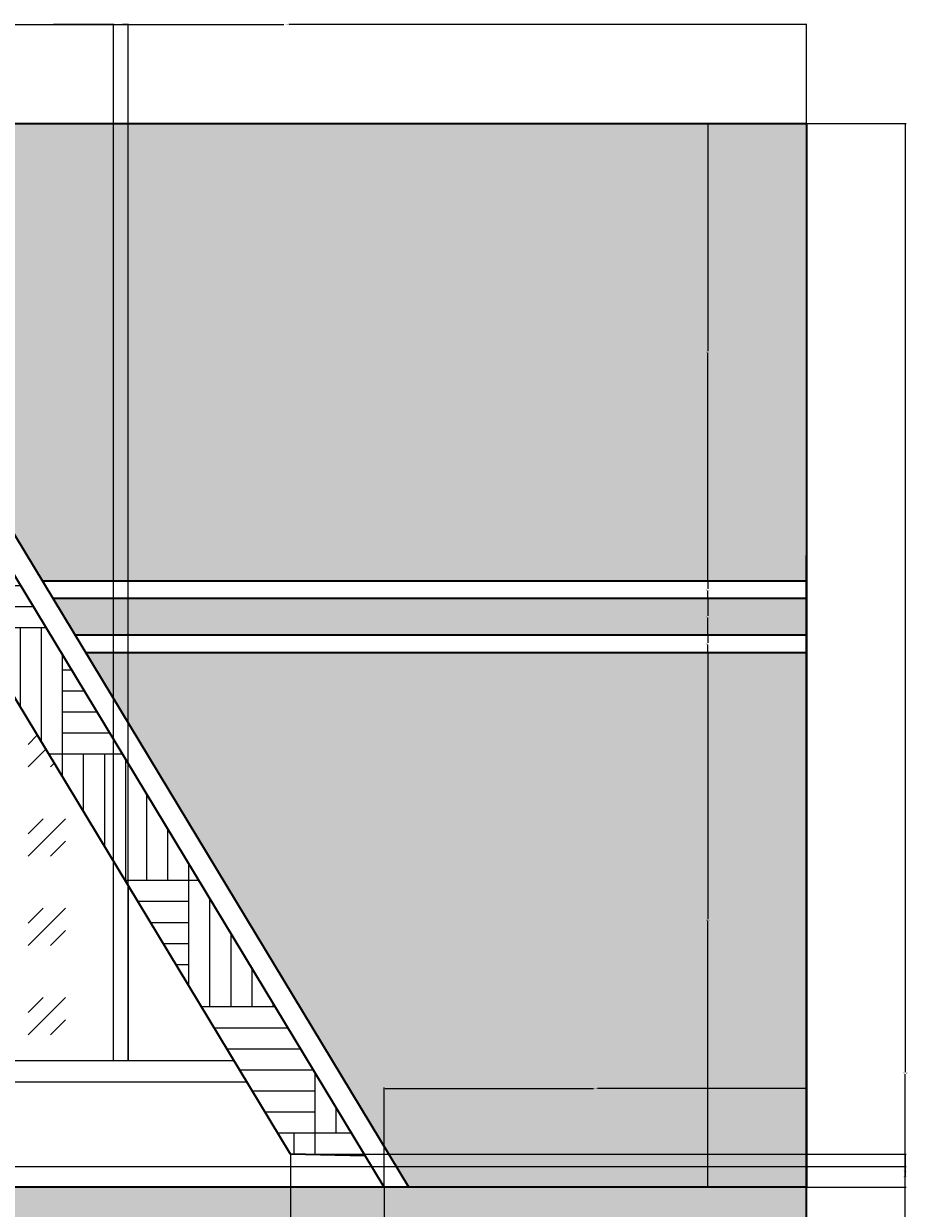
# Model space of a CAD drawing. Units: inches. Extents: x -9 to 389, y -55 to 344.
# Tile 5 of 5: x 221 to 389, y 119 to 344. Entities that reach past the tile are written whole.
import ezdxf

# ---------------------------------------------------------------- set-up
doc = ezdxf.new("R2010")
doc.units = ezdxf.units.IN
doc.header["$MEASUREMENT"] = 0
for name, color, linetype, lineweight in [('A-ANNO-DIMS', 2, 'Continuous', 18), ('A-ELEV', 7, 'Continuous', 35), ('A-ELEV-PATT', 8, 'Continuous', 13), ('A-GLAZ', 4, 'Continuous', 25), ('A-GLAZ-PATT', 252, 'Continuous', 13), ('A-ROOF', 1, 'Continuous', 35), ('A-ROOF-PATT', 8, 'Continuous', 13)]:
    doc.layers.add(name, color=color, linetype=linetype, lineweight=lineweight)
doc.styles.get("Standard").update_dxf_attribs({"font": 'arial.ttf'})
doc.dimstyles.get("Standard").update_dxf_attribs({"dimtxt": 0.18, "dimasz": 0.18, "dimexe": 0.18, "dimexo": 0.0625, "dimgap": 0.09, "dimtad": 0, "dimtih": 1, "dimtoh": 1, "dimdec": 4, "dimzin": 0, "dimdsep": 46, "dimtxsty": 'Standard', "dimcen": 0.09, "dimadec": 0, "dimazin": 0, "dimtfac": 1, "dimtdec": 4, "dimtofl": 0, "dimtmove": 0, "dimatfit": 3, "dimfxl": 1, "dimtolj": 1, "dimtzin": 0, "dimarcsym": 0})

# ---------------------------------------------------------------- blocks, each defined once
blk = doc.blocks.new('*D6')
at = {"layer": 'A-ANNO-DIMS', "color": 0, "lineweight": -2, "transparency": 16777216}
for p, q in [((171.93, 324.93), (171.93, 343.8)), ((172.11, 343.62), (270.34, 343.62)), ((369.47, 343.62), (271.25, 343.62)), ((369.65, 324.93), (369.65, 343.8))]:
    blk.add_line(p, q, dxfattribs=at)
at = {"layer": 'A-ANNO-DIMS', "color": 0, "transparency": 16777216}
for points in [[(172.11, 343.65), (172.11, 343.59), (171.93, 343.62)], [(369.47, 343.65), (369.47, 343.59), (369.65, 343.62)]]:
    blk.add_solid(points, dxfattribs=at)
at = {"layer": 'Defpoints', "color": 0, "transparency": 16777216}
for p in [(369.65, 343.62), (171.93, 324.87), (369.65, 324.87)]:
    blk.add_point(p, dxfattribs=at)
at = {"layer": 'A-ANNO-DIMS', "color": 0, "transparency": 16777216, "insert": (270.79, 343.62), "char_height": 0.18, "attachment_point": 5}
blk.add_mtext('\\A1;197.72', dxfattribs=at)
blk = doc.blocks.new('*D20')
at = {"layer": 'A-ANNO-DIMS', "color": 0, "lineweight": -2, "transparency": 16777216}
for p, q in [((369.72, 324.87), (388.58, 324.87)), ((388.4, 324.69), (388.4, 144.62)), ((388.4, -35.81), (388.4, 144.26)), ((146.92, -35.99), (388.58, -35.99))]:
    blk.add_line(p, q, dxfattribs=at)
at = {"layer": 'A-ANNO-DIMS', "color": 0, "transparency": 16777216}
for points in [[(388.37, 324.69), (388.43, 324.69), (388.4, 324.87)], [(388.37, -35.81), (388.43, -35.81), (388.4, -35.99)]]:
    blk.add_solid(points, dxfattribs=at)
at = {"layer": 'Defpoints', "color": 0, "transparency": 16777216}
for p in [(369.65, 324.87), (388.4, 324.87), (146.86, -35.99)]:
    blk.add_point(p, dxfattribs=at)
at = {"layer": 'A-ANNO-DIMS', "color": 0, "transparency": 16777216, "insert": (388.4, 144.44), "char_height": 0.18, "attachment_point": 5}
blk.add_mtext('\\A1;360.86', dxfattribs=at)
blk = doc.blocks.new('*D29')
at = {"layer": 'A-ANNO-DIMS', "color": 0, "lineweight": -2, "transparency": 16777216}
for p, q in [((369.59, 324.87), (-9.28, 324.87)), ((-9.1, 324.69), (-9.1, 319.05)), ((-9.1, 313.05), (-9.1, 318.69)), ((160.42, 312.87), (-9.28, 312.87))]:
    blk.add_line(p, q, dxfattribs=at)
at = {"layer": 'A-ANNO-DIMS', "color": 0, "transparency": 16777216}
for points in [[(-9.13, 324.69), (-9.07, 324.69), (-9.1, 324.87)], [(-9.13, 313.05), (-9.07, 313.05), (-9.1, 312.87)]]:
    blk.add_solid(points, dxfattribs=at)
at = {"layer": 'Defpoints', "color": 0, "transparency": 16777216}
for p in [(-9.1, 324.87), (369.65, 324.87), (160.49, 312.87)]:
    blk.add_point(p, dxfattribs=at)
at = {"layer": 'A-ANNO-DIMS', "color": 0, "transparency": 16777216, "insert": (-9.1, 318.87), "char_height": 0.18, "attachment_point": 5}
blk.add_mtext('\\A1;12', dxfattribs=at)
blk = doc.blocks.new('*D33')
at = {"layer": 'A-ANNO-DIMS', "color": 0, "lineweight": -2, "transparency": 16777216}
for p, q in [((289.4, 122.83), (289.4, 141.7)), ((289.58, 141.52), (329.13, 141.52)), ((369.47, 141.52), (329.92, 141.52)), ((369.65, 122.83), (369.65, 141.7))]:
    blk.add_line(p, q, dxfattribs=at)
at = {"layer": 'A-ANNO-DIMS', "color": 0, "transparency": 16777216}
for points in [[(289.58, 141.55), (289.58, 141.49), (289.4, 141.52)], [(369.47, 141.55), (369.47, 141.49), (369.65, 141.52)]]:
    blk.add_solid(points, dxfattribs=at)
at = {"layer": 'Defpoints', "color": 0, "transparency": 16777216}
for p in [(369.65, 141.52), (289.4, 122.77), (369.65, 122.77)]:
    blk.add_point(p, dxfattribs=at)
at = {"layer": 'A-ANNO-DIMS', "color": 0, "transparency": 16777216, "insert": (329.52, 141.52), "char_height": 0.18, "attachment_point": 5}
blk.add_mtext('\\A1;80.26', dxfattribs=at)
blk = doc.blocks.new('*D40')
at = {"layer": 'A-ANNO-DIMS', "color": 0, "lineweight": -2, "transparency": 16777216}
for p, q in [((369.59, 224.31), (350.72, 224.31)), ((350.9, 224.13), (350.9, 173.72)), ((350.9, 122.95), (350.9, 173.36)), ((369.59, 122.77), (350.72, 122.77))]:
    blk.add_line(p, q, dxfattribs=at)
at = {"layer": 'A-ANNO-DIMS', "color": 0, "transparency": 16777216}
for points in [[(350.87, 224.13), (350.93, 224.13), (350.9, 224.31)], [(350.87, 122.95), (350.93, 122.95), (350.9, 122.77)]]:
    blk.add_solid(points, dxfattribs=at)
at = {"layer": 'Defpoints', "color": 0, "transparency": 16777216}
for p in [(350.9, 224.31), (369.65, 224.31), (369.65, 122.77)]:
    blk.add_point(p, dxfattribs=at)
at = {"layer": 'A-ANNO-DIMS', "color": 0, "transparency": 16777216, "insert": (350.9, 173.54), "char_height": 0.18, "attachment_point": 5}
blk.add_mtext('\\A1;101.55', dxfattribs=at)
blk = doc.blocks.new('*D41')
at = {"layer": 'A-ANNO-DIMS', "color": 0, "lineweight": -2, "transparency": 16777216}
for p, q in [((369.59, 227.7), (350.72, 227.7)), ((350.9, 227.52), (350.9, 226.19)), ((350.9, 224.49), (350.9, 225.83)), ((369.59, 224.31), (350.72, 224.31))]:
    blk.add_line(p, q, dxfattribs=at)
at = {"layer": 'A-ANNO-DIMS', "color": 0, "transparency": 16777216}
for points in [[(350.87, 227.52), (350.93, 227.52), (350.9, 227.7)], [(350.87, 224.49), (350.93, 224.49), (350.9, 224.31)]]:
    blk.add_solid(points, dxfattribs=at)
at = {"layer": 'Defpoints', "color": 0, "transparency": 16777216}
for p in [(350.9, 227.7), (369.65, 227.7), (369.65, 224.31)]:
    blk.add_point(p, dxfattribs=at)
at = {"layer": 'A-ANNO-DIMS', "color": 0, "transparency": 16777216, "insert": (350.9, 226.01), "char_height": 0.18, "attachment_point": 5}
blk.add_mtext('\\A1;3.388', dxfattribs=at)
blk = doc.blocks.new('*D42')
at = {"layer": 'A-ANNO-DIMS', "color": 0, "lineweight": -2, "transparency": 16777216}
for p, q in [((369.59, 234.59), (350.72, 234.59)), ((350.9, 234.41), (350.9, 231.33)), ((350.9, 227.88), (350.9, 230.96)), ((369.59, 227.7), (350.72, 227.7))]:
    blk.add_line(p, q, dxfattribs=at)
at = {"layer": 'A-ANNO-DIMS', "color": 0, "transparency": 16777216}
for points in [[(350.87, 234.41), (350.93, 234.41), (350.9, 234.59)], [(350.87, 227.88), (350.93, 227.88), (350.9, 227.7)]]:
    blk.add_solid(points, dxfattribs=at)
at = {"layer": 'Defpoints', "color": 0, "transparency": 16777216}
for p in [(350.9, 234.59), (369.65, 234.59), (369.65, 227.7)]:
    blk.add_point(p, dxfattribs=at)
at = {"layer": 'A-ANNO-DIMS', "color": 0, "transparency": 16777216, "insert": (350.9, 231.15), "char_height": 0.18, "attachment_point": 5}
blk.add_mtext('\\A1;6.886', dxfattribs=at)
blk = doc.blocks.new('*D43')
at = {"layer": 'A-ANNO-DIMS', "color": 0, "lineweight": -2, "transparency": 16777216}
for p, q in [((369.59, 237.98), (350.72, 237.98)), ((350.9, 237.8), (350.9, 236.47)), ((369.59, 234.59), (350.72, 234.59)), ((350.9, 234.77), (350.9, 236.1))]:
    blk.add_line(p, q, dxfattribs=at)
at = {"layer": 'A-ANNO-DIMS', "color": 0, "transparency": 16777216}
for points in [[(350.87, 237.8), (350.93, 237.8), (350.9, 237.98)], [(350.87, 234.77), (350.93, 234.77), (350.9, 234.59)]]:
    blk.add_solid(points, dxfattribs=at)
at = {"layer": 'Defpoints', "color": 0, "transparency": 16777216}
for p in [(350.9, 237.98), (369.65, 237.98), (369.65, 234.59)]:
    blk.add_point(p, dxfattribs=at)
at = {"layer": 'A-ANNO-DIMS', "color": 0, "transparency": 16777216, "insert": (350.9, 236.28), "char_height": 0.18, "attachment_point": 5}
blk.add_mtext('\\A1;3.388', dxfattribs=at)
blk = doc.blocks.new('*D44')
at = {"layer": 'A-ANNO-DIMS', "color": 0, "lineweight": -2, "transparency": 16777216}
for p, q in [((369.59, 324.87), (350.72, 324.87)), ((350.9, 324.69), (350.9, 281.61)), ((350.9, 238.16), (350.9, 281.24)), ((369.59, 237.98), (350.72, 237.98))]:
    blk.add_line(p, q, dxfattribs=at)
at = {"layer": 'A-ANNO-DIMS', "color": 0, "transparency": 16777216}
for points in [[(350.87, 324.69), (350.93, 324.69), (350.9, 324.87)], [(350.87, 238.16), (350.93, 238.16), (350.9, 237.98)]]:
    blk.add_solid(points, dxfattribs=at)
at = {"layer": 'Defpoints', "color": 0, "transparency": 16777216}
for p in [(350.9, 324.87), (369.65, 324.87), (369.65, 237.98)]:
    blk.add_point(p, dxfattribs=at)
at = {"layer": 'A-ANNO-DIMS', "color": 0, "transparency": 16777216, "insert": (350.9, 281.42), "char_height": 0.18, "attachment_point": 5}
blk.add_mtext('\\A1;86.9', dxfattribs=at)
blk = doc.blocks.new('*D62')
at = {"layer": 'A-ANNO-DIMS', "color": 0, "lineweight": -2, "transparency": 16777216}
for p, q in [((214.29, 146.83), (214.29, 343.8)), ((214.47, 343.62), (225.66, 343.62)), ((237.78, 343.62), (226.59, 343.62)), ((237.96, 146.83), (237.96, 343.8))]:
    blk.add_line(p, q, dxfattribs=at)
at = {"layer": 'A-ANNO-DIMS', "color": 0, "transparency": 16777216}
for points in [[(214.47, 343.65), (214.47, 343.59), (214.29, 343.62)], [(237.78, 343.65), (237.78, 343.59), (237.96, 343.62)]]:
    blk.add_solid(points, dxfattribs=at)
at = {"layer": 'Defpoints', "color": 0, "transparency": 16777216}
for p in [(237.96, 343.62), (214.29, 146.77), (237.96, 146.77)]:
    blk.add_point(p, dxfattribs=at)
at = {"layer": 'A-ANNO-DIMS', "color": 0, "transparency": 16777216, "insert": (226.12, 343.62), "char_height": 0.18, "attachment_point": 5}
blk.add_mtext('\\A1;23.666', dxfattribs=at)
blk = doc.blocks.new('*D63')
at = {"layer": 'A-ANNO-DIMS', "color": 0, "lineweight": -2, "transparency": 16777216}
for p, q in [((237.96, 146.83), (237.96, 343.8)), ((238.14, 343.62), (239.02, 343.62)), ((240.55, 343.62), (239.67, 343.62)), ((240.73, 146.83), (240.73, 343.8))]:
    blk.add_line(p, q, dxfattribs=at)
at = {"layer": 'A-ANNO-DIMS', "color": 0, "transparency": 16777216}
for points in [[(238.14, 343.65), (238.14, 343.59), (237.96, 343.62)], [(240.55, 343.65), (240.55, 343.59), (240.73, 343.62)]]:
    blk.add_solid(points, dxfattribs=at)
at = {"layer": 'Defpoints', "color": 0, "transparency": 16777216}
for p in [(240.73, 343.62), (237.96, 146.77), (240.73, 146.77)]:
    blk.add_point(p, dxfattribs=at)
at = {"layer": 'A-ANNO-DIMS', "color": 0, "transparency": 16777216, "insert": (239.34, 343.62), "char_height": 0.18, "attachment_point": 5}
blk.add_mtext('\\A1;2.77', dxfattribs=at)
blk = doc.blocks.new('*D64')
at = {"layer": 'A-ANNO-DIMS', "color": 0, "lineweight": -2, "transparency": 16777216}
for p, q in [((130.27, 126.74), (388.58, 126.74)), ((388.4, 126.56), (388.4, 124.94)), ((388.4, 122.95), (388.4, 124.57)), ((118.84, 122.77), (388.58, 122.77))]:
    blk.add_line(p, q, dxfattribs=at)
at = {"layer": 'A-ANNO-DIMS', "color": 0, "transparency": 16777216}
for points in [[(388.37, 126.56), (388.43, 126.56), (388.4, 126.74)], [(388.37, 122.95), (388.43, 122.95), (388.4, 122.77)]]:
    blk.add_solid(points, dxfattribs=at)
at = {"layer": 'Defpoints', "color": 0, "transparency": 16777216}
for p in [(130.2, 126.74), (388.4, 126.74), (118.78, 122.77)]:
    blk.add_point(p, dxfattribs=at)
at = {"layer": 'A-ANNO-DIMS', "color": 0, "transparency": 16777216, "insert": (388.4, 124.76), "char_height": 0.18, "attachment_point": 5}
blk.add_mtext('\\A1;3.976', dxfattribs=at)
blk = doc.blocks.new('*D66')
at = {"layer": 'A-ANNO-DIMS', "color": 0, "lineweight": -2, "transparency": 16777216}
for p, q in [((271.64, 129.05), (388.58, 129.05)), ((388.4, 128.87), (388.4, 126.09)), ((388.4, 122.95), (388.4, 125.73)), ((289.46, 122.77), (388.58, 122.77))]:
    blk.add_line(p, q, dxfattribs=at)
at = {"layer": 'A-ANNO-DIMS', "color": 0, "transparency": 16777216}
for points in [[(388.37, 128.87), (388.43, 128.87), (388.4, 129.05)], [(388.37, 122.95), (388.43, 122.95), (388.4, 122.77)]]:
    blk.add_solid(points, dxfattribs=at)
at = {"layer": 'Defpoints', "color": 0, "transparency": 16777216}
for p in [(271.58, 129.05), (289.4, 122.77), (388.4, 122.77)]:
    blk.add_point(p, dxfattribs=at)
at = {"layer": 'A-ANNO-DIMS', "color": 0, "transparency": 16777216, "insert": (388.4, 125.91), "char_height": 0.18, "attachment_point": 5}
blk.add_mtext('\\A1;6.281', dxfattribs=at)
blk = doc.blocks.new('*D67')
at = {"layer": 'A-ANNO-DIMS', "color": 0, "lineweight": -2, "transparency": 16777216}
for p, q in [((271.58, 128.99), (271.58, -54.92)), ((289.4, 122.71), (289.4, -54.92)), ((271.76, -54.74), (280.03, -54.74)), ((289.22, -54.74), (280.94, -54.74))]:
    blk.add_line(p, q, dxfattribs=at)
at = {"layer": 'A-ANNO-DIMS', "color": 0, "transparency": 16777216}
for points in [[(271.76, -54.71), (271.76, -54.77), (271.58, -54.74)], [(289.22, -54.71), (289.22, -54.77), (289.4, -54.74)]]:
    blk.add_solid(points, dxfattribs=at)
at = {"layer": 'Defpoints', "color": 0, "transparency": 16777216}
for p in [(271.58, 129.05), (289.4, 122.77), (289.4, -54.74)]:
    blk.add_point(p, dxfattribs=at)
at = {"layer": 'A-ANNO-DIMS', "color": 0, "transparency": 16777216, "insert": (280.49, -54.74), "char_height": 0.18, "attachment_point": 5}
blk.add_mtext('\\A1;17.817', dxfattribs=at)
blk = doc.blocks.new('*D68')
at = {"layer": 'A-ANNO-DIMS', "color": 0, "lineweight": -2, "transparency": 16777216}
for p, q in [((114.32, 122.71), (114.32, -54.92)), ((289.4, 122.71), (289.4, -54.92)), ((114.5, -54.74), (201.4, -54.74)), ((289.22, -54.74), (202.31, -54.74))]:
    blk.add_line(p, q, dxfattribs=at)
at = {"layer": 'A-ANNO-DIMS', "color": 0, "transparency": 16777216}
for points in [[(114.5, -54.71), (114.5, -54.77), (114.32, -54.74)], [(289.22, -54.71), (289.22, -54.77), (289.4, -54.74)]]:
    blk.add_solid(points, dxfattribs=at)
at = {"layer": 'Defpoints', "color": 0, "transparency": 16777216}
for p in [(114.32, 122.77), (289.4, 122.77), (289.4, -54.74)]:
    blk.add_point(p, dxfattribs=at)
at = {"layer": 'A-ANNO-DIMS', "color": 0, "transparency": 16777216, "insert": (201.86, -54.74), "char_height": 0.18, "attachment_point": 5}
blk.add_mtext('\\A1;175.08', dxfattribs=at)

msp = doc.modelspace()

# ---------------------------------------------------------------- hatches: boundary and pattern name
at = {"layer": 'A-ELEV-PATT'}
h = msp.add_hatch(color=256, dxfattribs=at)
h.dxf.hatch_style = 1
h.paths.add_polyline_path([(369.6533, 324.8713), (171.9292, 324.8713), (224.4434, 237.9774), (369.6533, 237.9774)])
h.paths.add_polyline_path([(369.6533, 224.3149), (232.7004, 224.3149), (294.07, 122.7681), (369.6533, 122.7681)])
h = msp.add_hatch(color=256, dxfattribs=at)
h.dxf.hatch_style = 1
h.paths.add_polyline_path([(369.6533, 234.5893), (226.491, 234.5893), (230.6528, 227.703), (369.6533, 227.703)])
h = msp.add_hatch(color=256, dxfattribs=at)
h.dxf.hatch_style = 1
h.paths.add_polyline_path([(369.6533, 122.7681), (289.3963, 122.7681), (9.6533, 122.7681), (9.6533, 2.7681), (369.6533, 2.7681)])
h.paths.add_polyline_path([(177.6533, 110.7681), (177.6533, 14.7681), (21.6533, 14.7681), (21.6533, 110.7681)], flags=16)
h.paths.add_polyline_path([(201.6533, 110.7681), (357.6533, 110.7681), (357.6533, 14.7681), (201.6533, 14.7681)], flags=16)
h.paths.add_polyline_path([(156.7573, 110.7681), (156.7573, 14.7681), (153.9877, 14.7681), (153.9877, 110.7681)], flags=0)
h.paths.add_polyline_path([(222.5492, 110.7681), (225.3188, 110.7681), (225.3188, 14.7681), (222.5492, 14.7681)], flags=0)
h.paths.add_polyline_path([(246.2148, 110.7681), (248.9844, 110.7681), (248.9844, 14.7681), (246.2148, 14.7681)], flags=0)
h.paths.add_polyline_path([(269.8803, 110.7681), (272.65, 110.7681), (272.65, 14.7681), (269.8803, 14.7681)], flags=0)
h.paths.add_polyline_path([(68.9844, 110.7681), (68.9844, 14.7681), (66.2148, 14.7681), (66.2148, 110.7681)], flags=0)
h.paths.add_polyline_path([(45.3188, 110.7681), (45.3188, 14.7681), (42.5492, 14.7681), (42.5492, 110.7681)], flags=0)
at = {"layer": 'A-GLAZ-PATT', "transparency": 33554536}
h = msp.add_hatch(dxfattribs=at)
h.set_pattern_fill('GOST_GLASS', color=256, scale=2)
h.set_pattern_definition([(45, (-83.729, -34.93), (16.97056, 0), [10, -14]), (45, (-79.486, -34.93), (16.97056, 0), [4, -20]), (45, (-83.729, -30.687), (16.97056, 0), [4, -20])])
h.paths.add_polyline_path([(153.9877, 110.7681), (68.9844, 110.7681), (68.9844, 14.7681), (153.9877, 14.7681)])
h.paths.add_polyline_path([(357.6533, 110.7681), (272.65, 110.7681), (272.65, 14.7681), (357.6533, 14.7681)])
h.paths.add_polyline_path([(190.6266, 218.7681), (169.7307, 218.7681), (169.7307, 146.7681), (190.6266, 146.7681)])
h.paths.add_polyline_path([(143.2954, 218.7681), (122.3995, 218.7681), (122.3995, 146.7681), (143.2954, 146.7681)])
h.paths.add_polyline_path([(237.9578, 184.6816), (217.3576, 218.7681), (217.0618, 218.7681), (217.0618, 146.7681), (237.9578, 146.7681)])
h.paths.add_polyline_path([(42.5492, 110.7681), (21.6533, 110.7681), (21.6533, 14.7681), (42.5492, 14.7681)])
h.paths.add_polyline_path([(246.2148, 110.7681), (225.3188, 110.7681), (225.3188, 14.7681), (246.2148, 14.7681)])
at = {"layer": 'A-ROOF-PATT'}
h = msp.add_hatch(dxfattribs=at)
h.set_pattern_fill('AR-PARQ1', color=256, scale=2)
h.set_pattern_definition([(90, (-83.73, -34.93), (-24, 24), [24, -24]), (90, (-79.73, -34.93), (-24, 24), [24, -24]), (90, (-75.73, -34.93), (-24, 24), [24, -24]), (90, (-71.73, -34.93), (-24, 24), [24, -24]), (90, (-67.73, -34.93), (-24, 24), [24, -24]), (90, (-63.73, -34.93), (-24, 24), [24, -24]), (90, (-59.73, -34.93), (-24, 24), [24, -24]), (0, (-83.73, -10.93), (24, -24), [24, -24]), (0, (-83.73, -6.93), (24, -24), [24, -24]), (0, (-83.73, -2.93), (24, -24), [24, -24]), (0, (-83.73, 1.07), (24, -24), [24, -24]), (0, (-83.73, 5.07), (24, -24), [24, -24]), (0, (-83.73, 9.07), (24, -24), [24, -24]), (0, (-83.73, 13.07), (24, -24), [24, -24])])
h.paths.add_polyline_path([(59.2615, 270.2003), (45.8744, 270.2003), (116.6802, 127.0192), (130.2035, 126.7437)])
h.paths.add_polyline_path([(174.5076, 312.8713), (160.4864, 312.8713), (271.5791, 129.0492), (285.7644, 128.7778)])

# ---------------------------------------------------------------- linework, layer by layer
at = {"layer": 'A-ELEV'}
for p, q in [((369.6533, 324.8713), (369.6533, 122.7681)), ((369.6533, 2.7681), (369.6533, 242.7681)), ((369.6533, 122.7681), (9.6533, 122.7681)), ((369.6533, 122.7681), (289.3963, 122.7681))]:
    msp.add_line(p, q, dxfattribs=at)
for points in [[(224.4434, 237.9774), (369.6533, 237.9774), (369.6533, 234.5893), (226.491, 234.5893)], [(230.6528, 227.703), (369.6533, 227.703), (369.6533, 224.3149), (232.7004, 224.3149)]]:
    msp.add_lwpolyline(points, dxfattribs=at)
at = {"layer": 'A-GLAZ'}
for p, q in [((260.8707, 146.7681), (120.3011, 146.7681)), ((263.2881, 142.7681), (122.2791, 142.7681))]:
    msp.add_line(p, q, dxfattribs=at)
for points in [[(237.9578, 146.7681), (237.9578, 184.6816)], [(240.7274, 180.0987), (240.7274, 146.7681)], [(240.7274, 122.7681), (237.9578, 122.7681)]]:
    msp.add_lwpolyline(points, dxfattribs=at)
at = {"layer": 'A-ROOF'}
for p, q in [((289.3963, 122.7681), (167.2555, 324.8713)), ((167.2555, 324.8713), (369.6533, 324.8713)), ((294.07, 122.7681), (171.9292, 324.8713)), ((271.5791, 129.0492), (160.4864, 312.8713)), ((285.7644, 128.7778), (271.5791, 129.0492))]:
    msp.add_line(p, q, dxfattribs=at)

# ---------------------------------------------------------------- dimensions: what is measured, and where the dimension line sits
at = {"layer": 'A-ANNO-DIMS'}
for base, p1, p2, override, picture, middle in [((369.6533, 343.6213), (171.9292, 324.8713), (369.6533, 324.8713), {"dimdec": 2, "dimlfac": 1, "dimrnd": 0, "dimzin": 0, "dimdsep": 46, "dimlunit": 2}, '*D6', (270.7912, 343.6213)), ((237.9578, 343.6213), (214.2922, 146.7681), (237.9578, 146.7681), {"dimdec": 3, "dimlfac": 1, "dimrnd": 0, "dimzin": 0, "dimdsep": 46, "dimlunit": 2}, '*D62', (226.125, 343.6213)), ((240.7274, 343.6213), (237.9578, 146.7681), (240.7274, 146.7681), {"dimdec": 2, "dimlfac": 1, "dimrnd": 0, "dimzin": 0, "dimdsep": 46, "dimlunit": 2}, '*D63', (239.3426, 343.6213)), ((369.6533, 141.5181), (289.3963, 122.7681), (369.6533, 122.7681), {"dimdec": 2, "dimlfac": 1, "dimrnd": 0, "dimzin": 0, "dimdsep": 46, "dimlunit": 2}, '*D33', (329.5248, 141.5181)), ((289.3963, -54.7386), (271.5791, 129.0492), (289.3963, 122.7681), {"dimdec": 3, "dimlfac": 1, "dimrnd": 0, "dimzin": 0, "dimdsep": 46, "dimlunit": 2}, '*D67', (280.4877, -54.7386)), ((289.3963, -54.7386), (114.32, 122.7681), (289.3963, 122.7681), {"dimdec": 2, "dimlfac": 1, "dimrnd": 0, "dimzin": 0, "dimdsep": 46, "dimlunit": 2}, '*D68', (201.8582, -54.7386))]:
    dim = msp.add_linear_dim(base=base, p1=p1, p2=p2, dimstyle='Standard', override=override, dxfattribs=at)
    dim.commit()
    dim.dimension.update_dxf_attribs({"geometry": picture, "text_midpoint": middle})
for base, p1, p2, override, picture, middle in [((-9.0967, 324.8713), (160.4864, 312.8713), (369.6533, 324.8713), {"dimdec": 0, "dimlfac": 1, "dimrnd": 0, "dimzin": 0, "dimdsep": 46, "dimlunit": 2}, '*D29', (-9.0967, 318.8713)), ((388.4033, 324.8713), (146.8603, -35.9886), (369.6533, 324.8713), {"dimdec": 2, "dimlfac": 1, "dimrnd": 0, "dimzin": 0, "dimdsep": 46, "dimlunit": 2}, '*D20', (388.4033, 144.4414)), ((350.9033, 324.8713), (369.6533, 237.9774), (369.6533, 324.8713), {"dimdec": 1, "dimlfac": 1, "dimrnd": 0, "dimzin": 0, "dimdsep": 46, "dimlunit": 2}, '*D44', (350.9033, 281.4244)), ((350.9033, 237.9774), (369.6533, 234.5893), (369.6533, 237.9774), {"dimdec": 3, "dimlfac": 1, "dimrnd": 0, "dimzin": 0, "dimdsep": 46, "dimlunit": 2}, '*D43', (350.9033, 236.2833)), ((350.9033, 234.5893), (369.6533, 227.703), (369.6533, 234.5893), {"dimdec": 3, "dimlfac": 1, "dimrnd": 0, "dimzin": 0, "dimdsep": 46, "dimlunit": 2}, '*D42', (350.9033, 231.1462)), ((350.9033, 227.703), (369.6533, 224.3149), (369.6533, 227.703), {"dimdec": 3, "dimlfac": 1, "dimrnd": 0, "dimzin": 0, "dimdsep": 46, "dimlunit": 2}, '*D41', (350.9033, 226.009)), ((350.9033, 224.3149), (369.6533, 122.7681), (369.6533, 224.3149), {"dimdec": 2, "dimlfac": 1, "dimrnd": 0, "dimzin": 0, "dimdsep": 46, "dimlunit": 2}, '*D40', (350.9033, 173.5415)), ((388.4033, 122.7681), (271.5791, 129.0492), (289.3963, 122.7681), {"dimdec": 3, "dimlfac": 1, "dimrnd": 0, "dimzin": 0, "dimdsep": 46, "dimlunit": 2}, '*D66', (388.4033, 125.9087)), ((388.4033, 126.7437), (118.7824, 122.7681), (130.2035, 126.7437), {"dimdec": 3, "dimlfac": 1, "dimrnd": 0, "dimzin": 0, "dimdsep": 46, "dimlunit": 2}, '*D64', (388.4033, 124.7559))]:
    dim = msp.add_linear_dim(base=base, p1=p1, p2=p2, angle=90, dimstyle='Standard', override=override, dxfattribs=at)
    dim.commit()
    dim.dimension.update_dxf_attribs({"geometry": picture, "text_midpoint": middle})

doc.saveas('drawing.dxf')
